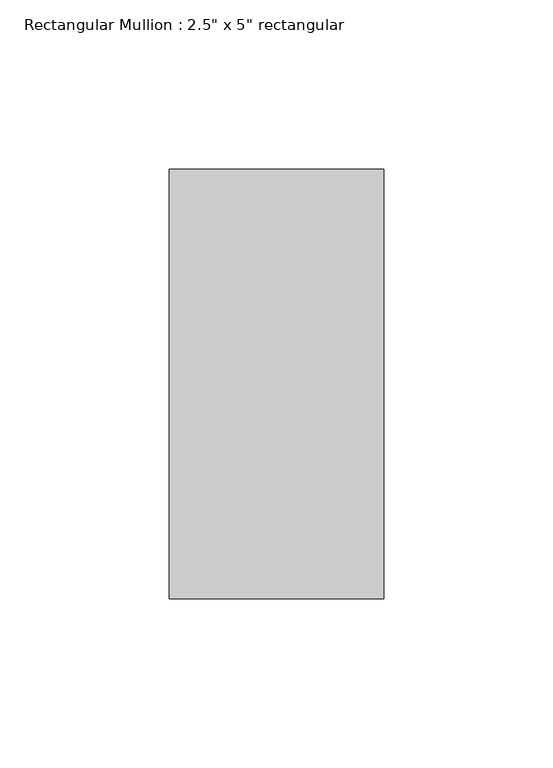
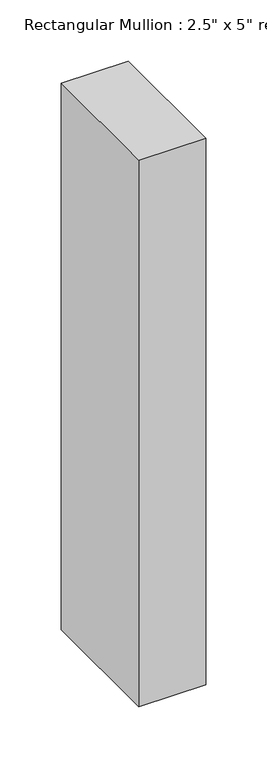
"""IFC4 building model written with IfcOpenShell, lengths in millimetres: member geometry."""

from ifc_helpers import new_model, si_unit, frame, origin, place, context, project, spatial, polyline, outline, extrude, source, transform, mapped, element, save


def member_0a1a1ade(model_context):
    return source(origin(), model_context, "Body", "SweptSolid", [
        extrude(outline(polyline([(31.75, 63.5), (31.75, -63.5), (-31.75, -63.5), (-31.75, 63.5), (31.75, 63.5)])), frame((0.0, 0.0, -546.1), z_axis=(0.0, 0.0, 1.0), x_axis=(1.0, 0.0, 0.0)), (0.0, 0.0, 1.0), 546.1),
    ])


if __name__ == "__main__":
    model = new_model("IFC4")
    model_context = context("Model", 3, world=origin())
    ifc_project = project(units=[si_unit("LENGTHUNIT", "METRE", prefix="MILLI")], contexts=[model_context])
    site = spatial("IfcSite", under=ifc_project)
    building = spatial("IfcBuilding", under=site)
    placement = place(None, origin())
    member_shape = member_0a1a1ade(model_context)
    element("IfcMember", 1, ObjectType="Rectangular Mullion : 2.5\" x 5\" rectangular", at=placement, inside=building, context=model_context, shape_type="MappedRepresentation", body=[
        mapped(member_shape, transform((0.0, 0.0, 0.0), x_axis=(1.0, 0.0, 0.0), y_axis=(0.0, 1.0, 0.0), z_axis=(0.0, 0.0, 1.0))),
    ])
    save(model, "model.ifc")

# Revit data of these elements
# Type "Rectangular Mullion : 2.5\" x 5\" rectangular"
#   built-in parameter 1007304 = 0.416667 (stored number, unit not read)
#   built-in parameter 1007301 = 0.104167 (stored number, unit not read)
#   built-in parameter 1007300 = 0.104167 (stored number, unit not read)
